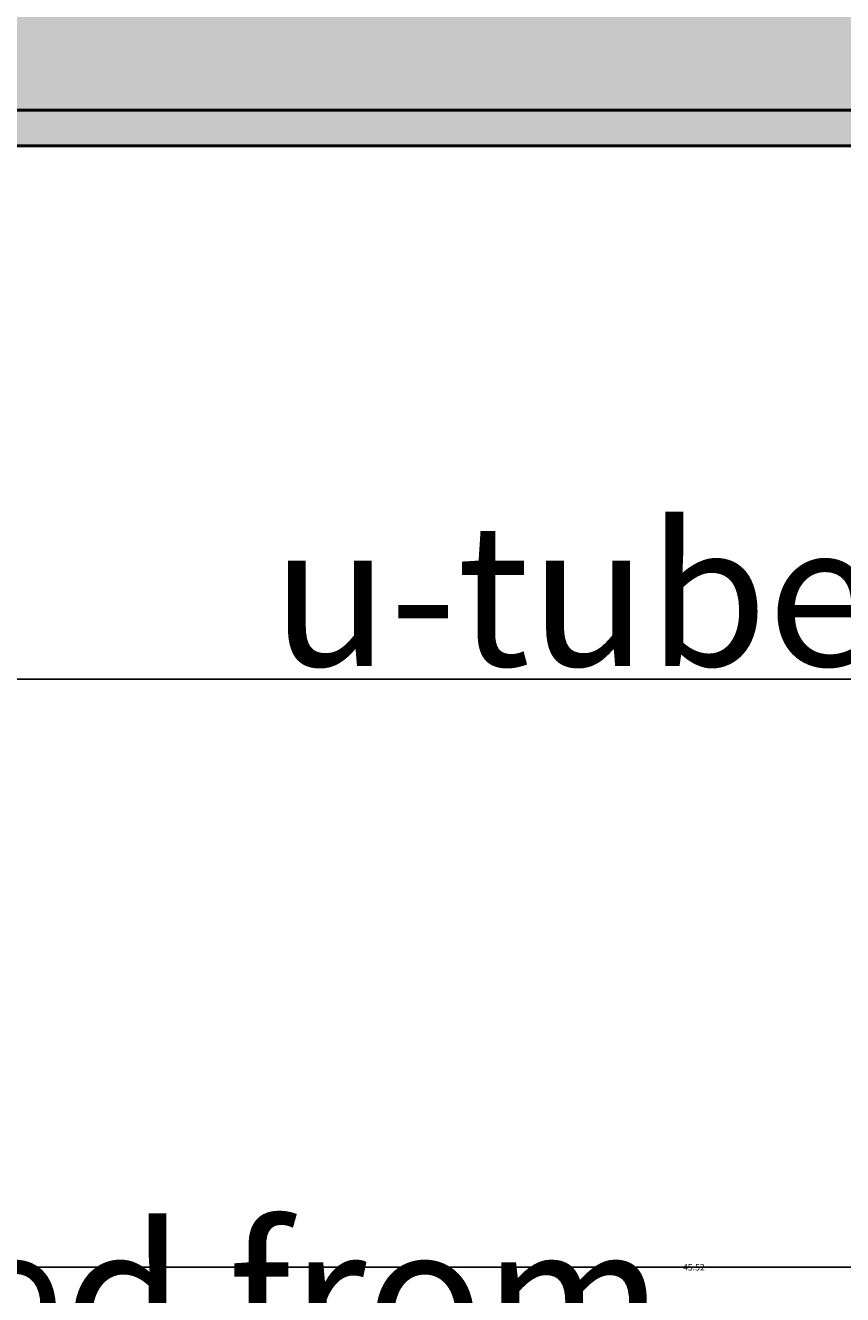
# Model space of a CAD drawing. Units: inches. Extents: x -12 to 334, y -10 to 186.
# Tile 34 of 77: x 175 to 198, y 14 to 49. Entities that reach past the tile are written whole.
import ezdxf
from ezdxf import colors
from ezdxf.entities.mleader import LeaderData, LeaderLine
from ezdxf.math import Vec2, Vec3

# ---------------------------------------------------------------- set-up
doc = ezdxf.new("R2010")
doc.units = ezdxf.units.IN
doc.header["$MEASUREMENT"] = 0
for name, color, linetype, lineweight in [('M-ANNO-TEXT', 3, 'Continuous', 25), ('M-DIMS', 2, 'Continuous', 18), ('M-EQPM', 7, 'Continuous', 50), ('M-EQPM-PATT', 8, 'Continuous', 18)]:
    doc.layers.add(name, color=color, linetype=linetype, lineweight=lineweight)
doc.styles.get("Standard").update_dxf_attribs({"font": 'arial.ttf'})
doc.dimstyles.get("Standard").update_dxf_attribs({"dimtxt": 0.18, "dimasz": 0.18, "dimexe": 0.18, "dimexo": 0.0625, "dimgap": 0.09, "dimtad": 0, "dimtih": 1, "dimtoh": 1, "dimdec": 4, "dimzin": 0, "dimdsep": 46, "dimtxsty": 'Standard', "dimcen": 0.09, "dimadec": 0, "dimazin": 0, "dimtfac": 1, "dimtdec": 4, "dimtofl": 0, "dimtmove": 0, "dimatfit": 3, "dimfxl": 1, "dimtolj": 1, "dimtzin": 0, "dimarcsym": 0})

# ---------------------------------------------------------------- blocks, each defined once
blk = doc.blocks.new('*D1')
at = {"layer": 'Defpoints', "color": 0, "transparency": 16777216}
for p in [(281.426, 91.899), (3.376, 80.692), (281.426, 14.304)]:
    blk.add_point(p, dxfattribs=at)
at = {"layer": 'M-DIMS', "color": 0, "lineweight": -2, "transparency": 16777216}
for p, q in [((281.426, 91.836), (281.426, 14.124)), ((3.376, 80.629), (3.376, 14.124)), ((3.556, 14.304), (141.935, 14.304)), ((281.246, 14.304), (142.867, 14.304))]:
    blk.add_line(p, q, dxfattribs=at)
at = {"layer": 'M-DIMS', "color": 0, "transparency": 16777216}
for points in [[(3.556, 14.334), (3.556, 14.274), (3.376, 14.304)], [(281.246, 14.334), (281.246, 14.274), (281.426, 14.304)]]:
    blk.add_solid(points, dxfattribs=at)
at = {"layer": 'M-DIMS', "color": 0, "transparency": 16777216, "insert": (142.401, 14.304), "char_height": 0.18, "attachment_point": 5}
blk.add_mtext('\\A1;278.05', dxfattribs=at)
blk = doc.blocks.new('*D29')
at = {"layer": 'Defpoints', "color": 0, "transparency": 16777216}
for p in [(-11.174, 45.854), (221.576, 45.854), (216.576, 30.854)]:
    blk.add_point(p, dxfattribs=at)
at = {"layer": 'M-DIMS', "color": 0, "lineweight": -2, "transparency": 16777216}
for p, q in [((221.514, 45.854), (-11.354, 45.854)), ((-11.174, 45.674), (-11.174, 38.536)), ((-11.174, 31.034), (-11.174, 38.172)), ((216.514, 30.854), (-11.354, 30.854))]:
    blk.add_line(p, q, dxfattribs=at)
at = {"layer": 'M-DIMS', "color": 0, "transparency": 16777216}
for points in [[(-11.204, 45.674), (-11.144, 45.674), (-11.174, 45.854)], [(-11.204, 31.034), (-11.144, 31.034), (-11.174, 30.854)]]:
    blk.add_solid(points, dxfattribs=at)
at = {"layer": 'M-DIMS', "color": 0, "transparency": 16777216, "insert": (-11.174, 38.354), "char_height": 0.18, "attachment_point": 5}
blk.add_mtext('\\A1;15', dxfattribs=at)
blk = doc.blocks.new('*D32')
at = {"layer": 'Defpoints', "color": 0, "transparency": 16777216}
for p in [(170.908, 61.105), (216.428, 61.105), (216.428, 14.304)]:
    blk.add_point(p, dxfattribs=at)
at = {"layer": 'M-DIMS', "color": 0, "lineweight": -2, "transparency": 16777216}
for p, q in [((170.908, 61.042), (170.908, 14.124)), ((216.428, 61.042), (216.428, 14.124)), ((171.088, 14.304), (193.271, 14.304)), ((216.248, 14.304), (194.064, 14.304))]:
    blk.add_line(p, q, dxfattribs=at)
at = {"layer": 'M-DIMS', "color": 0, "transparency": 16777216}
for points in [[(171.088, 14.334), (171.088, 14.274), (170.908, 14.304)], [(216.248, 14.334), (216.248, 14.274), (216.428, 14.304)]]:
    blk.add_solid(points, dxfattribs=at)
at = {"layer": 'M-DIMS', "color": 0, "transparency": 16777216, "insert": (193.668, 14.304), "char_height": 0.18, "attachment_point": 5}
blk.add_mtext('\\A1;45.52', dxfattribs=at)
blk = doc.blocks.new('*D39')
at = {"layer": 'Defpoints', "color": 0, "transparency": 16777216}
for p in [(279.726, 80.692), (-11.174, 45.854), (269.381, 45.854)]:
    blk.add_point(p, dxfattribs=at)
at = {"layer": 'M-DIMS', "color": 0, "lineweight": -2, "transparency": 16777216}
for p, q in [((279.664, 80.692), (-11.354, 80.692)), ((-11.174, 80.512), (-11.174, 63.455)), ((-11.174, 46.034), (-11.174, 63.091)), ((269.318, 45.854), (-11.354, 45.854))]:
    blk.add_line(p, q, dxfattribs=at)
at = {"layer": 'M-DIMS', "color": 0, "transparency": 16777216}
for points in [[(-11.204, 80.512), (-11.144, 80.512), (-11.174, 80.692)], [(-11.204, 46.034), (-11.144, 46.034), (-11.174, 45.854)]]:
    blk.add_solid(points, dxfattribs=at)
at = {"layer": 'M-DIMS', "color": 0, "transparency": 16777216, "insert": (-11.174, 63.273), "char_height": 0.18, "attachment_point": 5}
blk.add_mtext('\\A1;34.84', dxfattribs=at)

msp = doc.modelspace()

# ---------------------------------------------------------------- hatches: boundary and pattern name
at = {"layer": 'M-EQPM-PATT'}
h = msp.add_hatch(color=256, dxfattribs=at)
h.set_gradient(color1=(99, 100, 102), color2=(99, 100, 102), tint=1)
h.paths.add_polyline_path([(4.3766, 80.754, -0.4132606), (23.5807, 99.8958), (37.1002, 99.8958), (37.1002, 127.7078), (32.1002, 127.7078), (32.1002, 125.2078), (36.1002, 125.2078), (36.1002, 100.8958), (23.5807, 100.8958, 1), (23.5807, 60.4872), (36.1002, 60.4872), (36.1002, 36.1752), (32.1002, 36.1752), (32.1002, 33.6752), (37.1002, 33.6752), (37.1002, 61.4872), (23.5807, 61.4872, -0.384914), (4.4744, 78.754), (72.9244, 78.754), (72.9244, 69.6117), (75.9244, 69.6117), (75.9244, 89.8963), (72.9244, 89.8963), (72.9244, 80.754)])
h.paths.add_polyline_path([(54.1002, 125.2078), (58.1002, 125.2078), (58.1002, 127.7078), (53.1002, 127.7078), (53.1002, 99.8958), (64.5, 99.8958), (64.5, 109.0583), (63.5, 109.0583), (63.5, 100.8958), (54.1002, 100.8958)], flags=17)
h.paths.add_polyline_path([(53.1002, 33.6752), (58.1002, 33.6752), (58.1002, 36.1752), (54.1002, 36.1752), (54.1002, 60.4872), (64.2068, 60.4872), (64.2068, 49.4497), (87.8879, 49.4497), (87.8879, 55.3205), (104.8919, 55.3205), (104.8919, 30.8541), (99.8919, 30.8541), (99.8919, 28.8541), (105.8919, 28.8541), (105.8919, 56.3205), (87.8879, 56.3205), (87.8879, 63.6117), (86.8879, 63.6117), (86.8879, 50.4497), (65.0061, 50.4497), (65.0061, 63.6117), (64.5, 63.6117), (64.5, 61.4872), (53.1002, 61.4872)])
h.paths.add_polyline_path([(121.8919, 28.8541), (121.8919, 30.8541), (116.8919, 30.8541), (116.8919, 45.8541), (209.6965, 45.8541), (209.9204, 46.8541), (115.8919, 46.8541), (115.8919, 28.8541)])
h.paths.add_polyline_path([(221.5761, 32.8541), (216.5761, 32.8541), (216.5761, 30.8541), (222.5761, 30.8541), (222.5761, 46.8541), (209.9204, 46.8541), (209.6965, 45.8541), (221.5761, 45.8541)])
h.paths.add_polyline_path([(233.5761, 45.8541), (249.8485, 45.8541), (249.3759, 46.8541), (232.5761, 46.8541), (232.5761, 30.8541), (238.5761, 30.8541), (238.5761, 32.8541), (233.5761, 32.8541)])
h = msp.add_hatch(color=256, dxfattribs=at)
h.set_gradient(color1=(94, 103, 175), color2=(94, 103, 175), tint=1)
h.paths.add_polyline_path([(129.093, 89.8963), (86.8879, 89.8963), (86.8879, 69.6117), (129.093, 69.6117)], flags=17)
h.paths.add_polyline_path([(170.9079, 89.8963), (130.8573, 89.8963), (130.8573, 69.6117), (170.9079, 69.6117)], flags=17)
h.paths.add_polyline_path([(216.4278, 89.8963), (172.6722, 89.8963), (172.6722, 69.6117), (216.4278, 69.6117)], flags=17)
h.paths.add_polyline_path([(245.9354, 82.6969), (247.9354, 82.6969), (247.9354, 46.8541), (268.3808, 46.8541, 0.0998398), (279.7263, 80.6915), (251.9801, 80.6915, 0.4142136), (231.7758, 100.8958), (84.7229, 100.8958), (84.7229, 109.0583), (83.7229, 109.0583), (83.7229, 95.8963), (129.093, 95.8963), (129.093, 98.1081), (130.8573, 98.1081), (130.8573, 95.8963), (170.9079, 95.8963), (170.9079, 98.1081), (172.6722, 98.1081), (172.6722, 95.8963), (216.4278, 95.8963), (216.4278, 98.1081), (218.1922, 98.1081), (218.1922, 95.8963), (226.6083, 95.8963, -1), (226.6083, 63.6117), (218.1922, 63.6117), (218.1922, 61.1045), (216.4278, 61.1045), (216.4278, 63.6117), (172.6722, 63.6117), (172.6722, 61.1045), (170.9079, 61.1045), (170.9079, 63.6117), (130.8573, 63.6117), (130.8573, 61.1045), (129.093, 61.1045), (129.093, 63.6117), (87.8879, 63.6117), (87.8879, 56.3205), (105.8919, 56.3205), (105.8919, 28.8541), (115.8919, 28.8541), (115.8919, 46.8541), (222.5761, 46.8541), (222.5761, 30.8541), (232.5761, 30.8541), (232.5761, 46.8541), (245.9354, 46.8541)])
h.paths.add_polyline_path([(86.8879, 89.8963), (75.9244, 89.8963), (75.9244, 69.6117), (86.8879, 69.6117)])
h.paths.add_polyline_path([(83.7229, 109.0583), (75.9244, 109.0583), (75.9244, 95.8963), (83.7229, 95.8963)])
h.paths.add_polyline_path([(226.6083, 89.8963), (218.1922, 89.8963), (218.1922, 69.6117), (226.6083, 69.6117, 1)], flags=17)
h = msp.add_hatch(color=256, dxfattribs=at)
h.set_gradient(color1=(0, 0, 255), color2=(0, 0, 255), tint=1)
h.paths.add_polyline_path([(84.7229, 100.8958), (84.7229, 109.0583), (83.7229, 109.0583), (83.7229, 95.8963), (129.093, 95.8963), (129.093, 98.1081), (130.8573, 98.1081), (130.8573, 95.8963), (170.9079, 95.8963), (170.9079, 98.1081), (172.6722, 98.1081), (172.6722, 95.8963), (216.4278, 95.8963), (216.4278, 98.1081), (218.1922, 98.1081), (218.1922, 95.8963), (226.6083, 95.8963, -1), (226.6083, 63.6117), (218.1922, 63.6117), (218.1922, 61.1045), (216.4278, 61.1045), (216.4278, 63.6117), (172.6722, 63.6117), (172.6722, 61.1045), (170.9079, 61.1045), (170.9079, 63.6117), (130.8573, 63.6117), (130.8573, 61.1045), (129.093, 61.1045), (129.093, 63.6117), (87.8879, 63.6117), (87.8879, 56.3205), (105.8919, 56.3205), (105.8919, 28.8541), (115.8919, 28.8541), (115.8919, 46.8541), (222.5761, 46.8541), (222.5761, 30.8541), (232.5761, 30.8541), (232.5761, 46.8541), (245.9354, 46.8541), (245.9354, 82.6969), (247.9354, 82.6969), (247.9354, 46.8541), (268.3808, 46.8541, 0.0998398), (279.7263, 80.6915), (251.9801, 80.6915, 0.4142136), (231.7758, 100.8958)])

# ---------------------------------------------------------------- linework, layer by layer
at = {"layer": 'M-EQPM'}
for p, q in [((222.5761, 46.8541), (115.8919, 46.8541)), ((221.5761, 45.8541), (116.8919, 45.8541))]:
    msp.add_line(p, q, dxfattribs=at)

# ---------------------------------------------------------------- dimensions: what is measured, and where the dimension line sits
at = {"layer": 'M-DIMS'}
for base, p1, p2, picture, middle in [((281.4256, 14.3041), (3.3765, 80.6915), (281.4256, 91.8988), '*D1', (142.401, 14.3041)), ((216.4278, 14.3041), (170.9079, 61.1045), (216.4278, 61.1045), '*D32', (193.6678, 14.3041))]:
    dim = msp.add_linear_dim(base=base, p1=p1, p2=p2, dimstyle='Standard', override={"dimdec": 2, "dimlfac": 1, "dimrnd": 0, "dimzin": 0, "dimdsep": 46, "dimlunit": 2}, dxfattribs=at)
    dim.commit()
    dim.dimension.update_dxf_attribs({"geometry": picture, "text_midpoint": middle})
for p1, p2, override, picture, middle in [((279.7263, 80.6915), (269.3808, 45.8541), {"dimdec": 2, "dimlfac": 1, "dimrnd": 0, "dimzin": 0, "dimdsep": 46, "dimlunit": 2}, '*D39', (-11.1735, 63.2728)), ((216.5761, 30.8541), (221.5761, 45.8541), {"dimdec": 0, "dimlfac": 1, "dimrnd": 0, "dimzin": 0, "dimdsep": 46, "dimlunit": 2}, '*D29', (-11.1735, 38.3541))]:
    dim = msp.add_linear_dim(base=(-11.1736, 45.8541), p1=p1, p2=p2, angle=90, dimstyle='Standard', override=override, dxfattribs=at)
    dim.commit()
    dim.dimension.update_dxf_attribs({"geometry": picture, "text_midpoint": middle})

# ---------------------------------------------------------------- leaders
at = {"layer": 'M-ANNO-TEXT'}
ml = msp.add_multileader_mtext('Standard', dxfattribs=at)
ml.set_content('u-tubes', color=256)
ml.set_leader_properties()
ml.build(insert=Vec2(0, 0))
ml.multileader.update_dxf_attribs({"dogleg_length": 0.36, "arrow_head_size": 0.7})
ctx = ml.context
ctx.base_point, ctx.arrow_head_size, ctx.landing_gap_size, ctx.plane_origin = Vec3(183.1578, 33.1882), 0.7, 0.09, Vec3(168.0474, 30.6523)
ctx.text_align_type = 2
notes = []
notes.append((ctx, [(1, (1, 1, 0), (206.8598, 33.1882), (-1, 0), 5.4565, [(0, [(213.6735, 63.6117)], 0, [])])]))
ctx.mtext.insert, ctx.mtext.alignment, ctx.mtext.flow_direction = Vec3(201.3133, 35.2209), 3, 5
ml = msp.add_multileader_mtext('Standard', dxfattribs=at)
ml.set_content('liquid feed from\\Pcolumn', color=256)
ml.set_leader_properties()
ml.build(insert=Vec2(0, 0))
ml.multileader.update_dxf_attribs({"dogleg_length": 0.36, "arrow_head_size": 0.7})
ctx = ml.context
ctx.base_point, ctx.arrow_head_size, ctx.landing_gap_size, ctx.plane_origin = Vec3(152.1867, 13.4469), 0.7, 0.09, Vec3(117.7335, 28.8541)
notes.append((ctx, [(0, (1, 1, 0), (139.1325, 13.4469), (1, 0), 13.0542, [(0, [(117.7335, 28.8541)], 0, [])])]))
ctx.mtext.insert, ctx.mtext.flow_direction = Vec3(152.2767, 15.4796), 5
for ctx, leaders in notes:
    for number, flags, end, landing, length, lines in leaders:
        leader = LeaderData()
        leader.index, (leader.has_last_leader_line, leader.has_dogleg_vector, leader.attachment_direction) = number, flags
        leader.last_leader_point, leader.dogleg_vector, leader.dogleg_length = Vec3(end), Vec3(landing), length
        for number, points, colour, breaks in lines:
            line = LeaderLine()
            line.index, line.vertices, line.color, line.breaks = number, Vec3.list(points), colors.encode_raw_color(colour), breaks
            leader.lines.append(line)
        ctx.leaders.append(leader)

doc.saveas('drawing.dxf')
